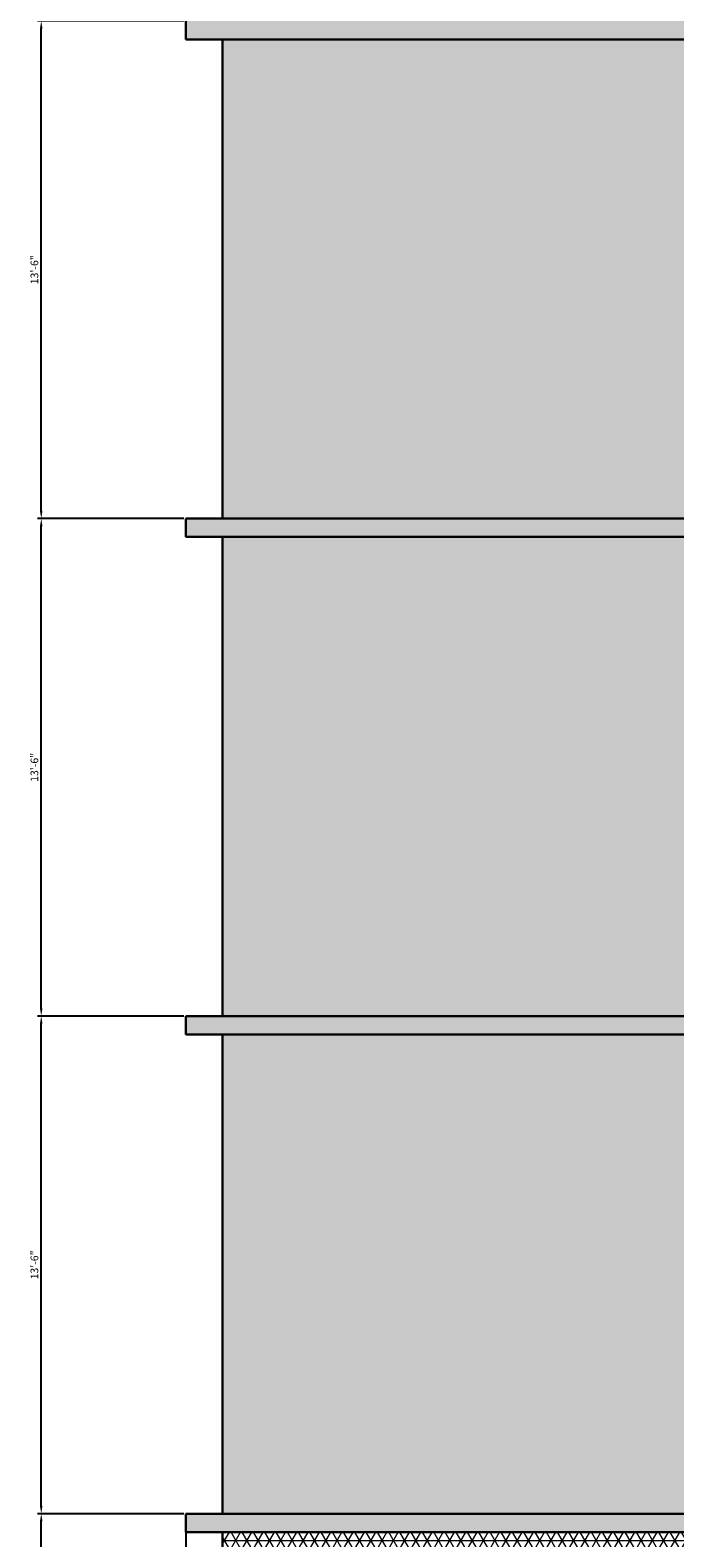
# Model space of a CAD drawing. Units: inches. Extents: x 2391 to 16591, y 7259 to 10239.
# Tile 8 of 27: x 2963 to 3173, y 7745 to 8236. Entities that reach past the tile are written whole.
import ezdxf

# ---------------------------------------------------------------- set-up
doc = ezdxf.new("R2010")
doc.units = ezdxf.units.IN
for name, color, linetype, lineweight in [('A-ANNO-DIMS', 4, 'Continuous', 18), ('A-ELEV', 7, 'Continuous', 30), ('A-ELEV-PATT', 8, 'Continuous', 13), ('A-ELEV-SURF-PATT', 253, 'Continuous', 13)]:
    doc.layers.add(name, color=color, linetype=linetype, lineweight=lineweight)
doc.styles.get("Standard").update_dxf_attribs({"font": 'arial.ttf'})
doc.dimstyles.new('ISO-25', dxfattribs={"dimtxt": 2.5, "dimasz": 2.5, "dimexe": 1.25, "dimexo": 0.625, "dimtad": 1, "dimdec": 0, "dimlunit": 3, "dimtxsty": 'Standard', "dimcen": 2.5, "dimadec": 0, "dimazin": 0, "dimtfac": 1, "dimtdec": 0, "dimtmove": 0, "dimatfit": 3, "dimfxl": 1, "dimarcsym": 0})

# ---------------------------------------------------------------- blocks, each defined once
blk = doc.blocks.new('*D83')
at = {"layer": 'A-ANNO-DIMS', "color": 0, "lineweight": -2, "transparency": 16777216}
for p, q in [((3013.78, 7751.89), (3013.78, 7528.22)), ((3469.78, 7751.89), (3469.78, 7528.22)), ((3016.28, 7529.47), (3467.28, 7529.47))]:
    blk.add_line(p, q, dxfattribs=at)
at = {"layer": 'A-ANNO-DIMS', "color": 0, "transparency": 16777216}
for points in [[(3016.28, 7529.89), (3016.28, 7529.05), (3013.78, 7529.47)], [(3467.28, 7529.89), (3467.28, 7529.05), (3469.78, 7529.47)]]:
    blk.add_solid(points, dxfattribs=at)
at = {"layer": 'Defpoints', "color": 0, "transparency": 16777216}
for p in [(3013.78, 7752.52), (3469.78, 7752.52), (3469.78, 7529.47)]:
    blk.add_point(p, dxfattribs=at)
at = {"layer": 'A-ANNO-DIMS', "color": 0, "transparency": 16777216, "insert": (3241.78, 7531.37), "char_height": 2.5, "attachment_point": 5}
blk.add_mtext('38\'-0"', dxfattribs=at)
blk = doc.blocks.new('*D85')
at = {"layer": 'A-ANNO-DIMS', "color": 0, "lineweight": -2, "transparency": 16777216}
for p, q in [((3013.15, 7752.52), (2965.48, 7752.52)), ((2966.73, 7579.02), (2966.73, 7750.02)), ((3019.15, 7576.52), (2965.48, 7576.52))]:
    blk.add_line(p, q, dxfattribs=at)
at = {"layer": 'A-ANNO-DIMS', "color": 0, "transparency": 16777216}
for points in [[(2966.31, 7750.02), (2967.14, 7750.02), (2966.73, 7752.52)], [(2966.31, 7579.02), (2967.14, 7579.02), (2966.73, 7576.52)]]:
    blk.add_solid(points, dxfattribs=at)
at = {"layer": 'Defpoints', "color": 0, "transparency": 16777216}
for p in [(2966.73, 7752.52), (3013.78, 7752.52), (3019.78, 7576.52)]:
    blk.add_point(p, dxfattribs=at)
at = {"layer": 'A-ANNO-DIMS', "color": 0, "transparency": 16777216, "insert": (2964.83, 7664.52), "char_height": 2.5, "attachment_point": 5, "rotation": 90}
blk.add_mtext('14\'-8"', dxfattribs=at)
blk = doc.blocks.new('*D86')
at = {"layer": 'A-ANNO-DIMS', "color": 0, "lineweight": -2, "transparency": 16777216}
for p, q in [((3013.15, 7914.52), (2965.48, 7914.52)), ((2966.73, 7755.02), (2966.73, 7912.02)), ((3013.15, 7752.52), (2965.48, 7752.52))]:
    blk.add_line(p, q, dxfattribs=at)
at = {"layer": 'A-ANNO-DIMS', "color": 0, "transparency": 16777216}
for points in [[(2966.31, 7912.02), (2967.14, 7912.02), (2966.73, 7914.52)], [(2966.31, 7755.02), (2967.14, 7755.02), (2966.73, 7752.52)]]:
    blk.add_solid(points, dxfattribs=at)
at = {"layer": 'Defpoints', "color": 0, "transparency": 16777216}
for p in [(2966.73, 7914.52), (3013.78, 7914.52), (3013.78, 7752.52)]:
    blk.add_point(p, dxfattribs=at)
at = {"layer": 'A-ANNO-DIMS', "color": 0, "transparency": 16777216, "insert": (2964.83, 7833.52), "char_height": 2.5, "attachment_point": 5, "rotation": 90}
blk.add_mtext('13\'-6"', dxfattribs=at)
blk = doc.blocks.new('*D87')
at = {"layer": 'A-ANNO-DIMS', "color": 0, "lineweight": -2, "transparency": 16777216}
for p, q in [((3013.15, 8076.52), (2965.48, 8076.52)), ((2966.73, 7917.02), (2966.73, 8074.02)), ((3013.15, 7914.52), (2965.48, 7914.52))]:
    blk.add_line(p, q, dxfattribs=at)
at = {"layer": 'A-ANNO-DIMS', "color": 0, "transparency": 16777216}
for points in [[(2966.31, 8074.02), (2967.14, 8074.02), (2966.73, 8076.52)], [(2966.31, 7917.02), (2967.14, 7917.02), (2966.73, 7914.52)]]:
    blk.add_solid(points, dxfattribs=at)
at = {"layer": 'Defpoints', "color": 0, "transparency": 16777216}
for p in [(2966.73, 8076.52), (3013.78, 8076.52), (3013.78, 7914.52)]:
    blk.add_point(p, dxfattribs=at)
at = {"layer": 'A-ANNO-DIMS', "color": 0, "transparency": 16777216, "insert": (2964.83, 7995.52), "char_height": 2.5, "attachment_point": 5, "rotation": 90}
blk.add_mtext('13\'-6"', dxfattribs=at)
blk = doc.blocks.new('*D88')
at = {"layer": 'A-ANNO-DIMS', "color": 0, "lineweight": -2, "transparency": 16777216}
for p, q in [((3013.15, 8238.52), (2965.48, 8238.52)), ((2966.73, 8079.02), (2966.73, 8236.02)), ((3013.15, 8076.52), (2965.48, 8076.52))]:
    blk.add_line(p, q, dxfattribs=at)
at = {"layer": 'A-ANNO-DIMS', "color": 0, "transparency": 16777216}
for points in [[(2966.31, 8236.02), (2967.14, 8236.02), (2966.73, 8238.52)], [(2966.31, 8079.02), (2967.14, 8079.02), (2966.73, 8076.52)]]:
    blk.add_solid(points, dxfattribs=at)
at = {"layer": 'Defpoints', "color": 0, "transparency": 16777216}
for p in [(2966.73, 8238.52), (3013.78, 8238.52), (3013.78, 8076.52)]:
    blk.add_point(p, dxfattribs=at)
at = {"layer": 'A-ANNO-DIMS', "color": 0, "transparency": 16777216, "insert": (2964.83, 8157.52), "char_height": 2.5, "attachment_point": 5, "rotation": 90}
blk.add_mtext('13\'-6"', dxfattribs=at)

msp = doc.modelspace()

# ---------------------------------------------------------------- hatches: boundary and pattern name
at = {"layer": 'A-ELEV-PATT'}
h = msp.add_hatch(dxfattribs=at)
h.set_pattern_fill('NET3', color=256)
h.paths.add_polyline_path([(3457.78, 8232.52), (3339.28, 8232.52), (3339.28, 8076.52), (3457.78, 8076.52)])
h.paths.add_polyline_path([(3415.03, 8124.52), (3373.03, 8124.52), (3373.03, 8178.52), (3415.03, 8178.52)], flags=16)
h.paths.add_polyline_path([(3412.03, 8127.52), (3376.03, 8127.52), (3376.03, 8175.52), (3412.03, 8175.52)], flags=0)
h.paths.add_polyline_path([(3457.78, 8070.52), (3339.28, 8070.52), (3339.28, 7914.52), (3457.78, 7914.52)])
h.paths.add_polyline_path([(3415.03, 7962.52), (3373.03, 7962.52), (3373.03, 8016.52), (3415.03, 8016.52)], flags=16)
h.paths.add_polyline_path([(3412.03, 7965.52), (3376.03, 7965.52), (3376.03, 8013.52), (3412.03, 8013.52)], flags=0)
h.paths.add_polyline_path([(3457.78, 7908.52), (3339.28, 7908.52), (3339.28, 7752.52), (3457.78, 7752.52)])
h.paths.add_polyline_path([(3415.03, 7800.52), (3373.03, 7800.52), (3373.03, 7854.52), (3415.03, 7854.52)], flags=16)
h.paths.add_polyline_path([(3412.03, 7803.52), (3376.03, 7803.52), (3376.03, 7851.52), (3412.03, 7851.52)], flags=0)
h.paths.add_polyline_path([(3339.28, 8232.52), (3227.28, 8232.52), (3227.28, 8076.52), (3339.28, 8076.52)])
h.paths.add_polyline_path([(3260.28, 8124.52), (3260.28, 8178.52), (3302.28, 8178.52), (3302.28, 8124.52)], flags=16)
h.paths.add_polyline_path([(3263.28, 8127.52), (3263.28, 8175.52), (3299.28, 8175.52), (3299.28, 8127.52)], flags=0)
h.paths.add_polyline_path([(3339.28, 8070.52), (3227.28, 8070.52), (3227.28, 7914.52), (3339.28, 7914.52)])
h.paths.add_polyline_path([(3260.28, 8016.52), (3302.28, 8016.52), (3302.28, 7962.52), (3260.28, 7962.52)], flags=16)
h.paths.add_polyline_path([(3263.28, 8013.52), (3299.28, 8013.52), (3299.28, 7965.52), (3263.28, 7965.52)], flags=0)
h.paths.add_polyline_path([(3339.28, 7908.52), (3227.28, 7908.52), (3227.28, 7752.52), (3339.28, 7752.52)])
h.paths.add_polyline_path([(3260.28, 7854.52), (3302.28, 7854.52), (3302.28, 7800.52), (3260.28, 7800.52)], flags=16)
h.paths.add_polyline_path([(3263.28, 7851.52), (3299.28, 7851.52), (3299.28, 7803.52), (3263.28, 7803.52)], flags=0)
h.paths.add_polyline_path([(3213.78, 7717.52), (3232.78, 7717.52), (3232.78, 7712.52), (3227.78, 7712.52), (3227.78, 7683.36), (3230.28, 7683.36), (3230.28, 7685.36), (3232.78, 7685.36), (3232.78, 7710.52), (3301.78, 7710.52), (3301.78, 7595.52), (3232.78, 7595.52), (3232.78, 7590.52), (3371.78, 7590.52), (3371.78, 7595.52), (3302.78, 7595.52), (3302.78, 7710.52), (3371.78, 7710.52), (3371.78, 7685.36), (3374.28, 7685.36), (3374.28, 7683.36), (3376.78, 7683.36), (3376.78, 7712.52), (3371.78, 7712.52), (3371.78, 7717.52), (3390.78, 7717.52), (3390.78, 7712.52), (3385.78, 7712.52), (3385.78, 7703.52), (3457.78, 7703.52), (3457.78, 7746.52), (3025.78, 7746.52), (3025.78, 7703.52), (3218.78, 7703.52), (3218.78, 7712.52), (3213.78, 7712.52)])
h.paths.add_polyline_path([(3232.78, 7679.36), (3230.28, 7679.36), (3230.28, 7681.36), (3227.78, 7681.36), (3227.78, 7623.23), (3230.28, 7623.23), (3230.28, 7625.23), (3232.78, 7625.23)], flags=17)
h.paths.add_polyline_path([(3232.78, 7619.23), (3230.28, 7619.23), (3230.28, 7621.23), (3227.78, 7621.23), (3227.78, 7590.52), (3232.78, 7590.52)], flags=17)
h.paths.add_polyline_path([(3376.78, 7681.36), (3374.28, 7681.36), (3374.28, 7679.36), (3371.78, 7679.36), (3371.78, 7625.23), (3374.28, 7625.23), (3374.28, 7623.23), (3376.78, 7623.23)], flags=17)
h.paths.add_polyline_path([(3376.78, 7621.23), (3374.28, 7621.23), (3374.28, 7619.23), (3371.78, 7619.23), (3371.78, 7590.52), (3376.78, 7590.52)], flags=17)
h = msp.add_hatch(dxfattribs=at)
h.set_pattern_fill('SQUARE', color=256)
h.paths.add_polyline_path([(3227.28, 8076.52), (3227.28, 8232.52), (3025.78, 8232.52), (3025.78, 8076.52)])
h.paths.add_polyline_path([(3178.28, 8160.52), (3178.28, 8178.52), (3208.28, 8178.52), (3208.28, 8160.52)], flags=16)
h.paths.add_polyline_path([(3181.28, 8163.52), (3181.28, 8175.52), (3205.28, 8175.52), (3205.28, 8163.52)], flags=0)
h.paths.add_polyline_path([(3025.78, 8070.52), (3025.78, 7914.52), (3227.28, 7914.52), (3227.28, 8070.52)])
h.paths.add_polyline_path([(3178.28, 7998.52), (3178.28, 8016.52), (3208.28, 8016.52), (3208.28, 7998.52)], flags=16)
h.paths.add_polyline_path([(3181.28, 8001.52), (3181.28, 8013.52), (3205.28, 8013.52), (3205.28, 8001.52)], flags=0)
h.paths.add_polyline_path([(3025.78, 7908.52), (3025.78, 7752.52), (3227.28, 7752.52), (3227.28, 7908.52)])
h.paths.add_polyline_path([(3178.28, 7854.52), (3208.28, 7854.52), (3208.28, 7836.52), (3178.28, 7836.52)], flags=16)
h.paths.add_polyline_path([(3181.28, 7851.52), (3205.28, 7851.52), (3205.28, 7839.52), (3181.28, 7839.52)], flags=0)
at = {"layer": 'A-ELEV-SURF-PATT'}
h = msp.add_hatch(color=256, dxfattribs=at)
h.dxf.hatch_style = 1
h.paths.add_polyline_path([(3469.78, 7746.52), (3469.78, 7752.52), (3013.78, 7752.52), (3013.78, 7746.52)])
h.paths.add_polyline_path([(3469.78, 7908.52), (3469.78, 7914.52), (3013.78, 7914.52), (3013.78, 7908.52)])
h.paths.add_polyline_path([(3469.78, 8070.52), (3469.78, 8076.52), (3013.78, 8076.52), (3013.78, 8070.52)])
h.paths.add_polyline_path([(3013.78, 8238.52), (3013.78, 8232.52), (3469.78, 8232.52), (3469.78, 8238.52)])
h.paths.add_polyline_path([(3236.28, 8339.52), (3236.28, 8334.52), (3436.78, 8334.52), (3436.78, 8339.52)])

# ---------------------------------------------------------------- linework, layer by layer
at = {"layer": 'A-ELEV'}
for p, q in [((3013.78, 8232.52), (3013.78, 8238.52)), ((3013.78, 8232.52), (3469.78, 8232.52)), ((3025.78, 8076.52), (3025.78, 8232.52)), ((3013.78, 8070.52), (3013.78, 8076.52)), ((3013.78, 8076.52), (3469.78, 8076.52)), ((3013.78, 8070.52), (3469.78, 8070.52)), ((3025.78, 7914.52), (3025.78, 8070.52)), ((3013.78, 7908.52), (3013.78, 7914.52)), ((3013.78, 7914.52), (3469.78, 7914.52)), ((3013.78, 7908.52), (3469.78, 7908.52)), ((3025.78, 7752.52), (3025.78, 7908.52)), ((3013.78, 7746.52), (3013.78, 7752.52)), ((3013.78, 7752.52), (3469.78, 7752.52)), ((3013.78, 7746.52), (3469.78, 7746.52)), ((3025.78, 7581.52), (3025.78, 7746.52))]:
    msp.add_line(p, q, dxfattribs=at)

# ---------------------------------------------------------------- dimensions: what is measured, and where the dimension line sits
at = {"layer": 'A-ANNO-DIMS'}
for base, p1, p2, picture, middle in [((2966.73, 8238.52), (3013.78, 8076.52), (3013.78, 8238.52), '*D88', (2964.83, 8157.52)), ((2966.73, 8076.52), (3013.78, 7914.52), (3013.78, 8076.52), '*D87', (2964.83, 7995.52)), ((2966.73, 7914.52), (3013.78, 7752.52), (3013.78, 7914.52), '*D86', (2964.83, 7833.52)), ((2966.73, 7752.52), (3019.78, 7576.52), (3013.78, 7752.52), '*D85', (2964.83, 7664.52))]:
    dim = msp.add_linear_dim(base=base, p1=p1, p2=p2, angle=90, dimstyle='ISO-25', override={"dimdec": 1, "dimlfac": 1, "dimrnd": 0, "dimzin": 1, "dimdsep": 46, "dimlunit": 4, "dimfrac": 2}, dxfattribs=at)
    dim.commit()
    dim.dimension.update_dxf_attribs({"geometry": picture, "text_midpoint": middle})
dim = msp.add_linear_dim(base=(3469.78, 7529.47), p1=(3013.78, 7752.52), p2=(3469.78, 7752.52), dimstyle='ISO-25', override={"dimdec": 1, "dimlfac": 1, "dimrnd": 0, "dimzin": 1, "dimdsep": 46, "dimlunit": 4, "dimfrac": 2}, dxfattribs=at)
dim.commit()
dim.dimension.update_dxf_attribs({"geometry": '*D83', "text_midpoint": (3241.78, 7531.37)})

doc.saveas('drawing.dxf')
